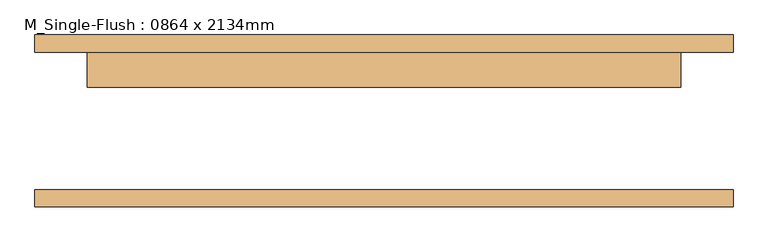
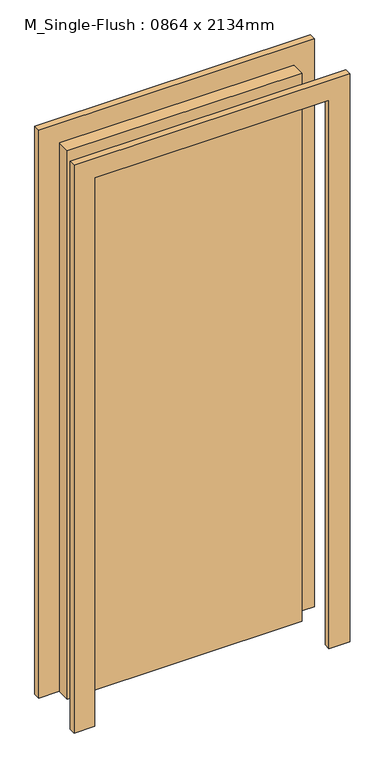
"""IFC4 building model written with IfcOpenShell, lengths in millimetres: door geometry, M_Single-Flush : 0864 x 2134mm."""

from ifc_helpers import new_model, si_unit, frame, origin, origin_with_axes, place, context, project, spatial, polyline, outline, extrude, source, transform, mapped, element, save


def m_single_flush_0864_x_2134mm_5c09ce2c(model_context):
    return source(origin(), model_context, "Body", "SweptSolid", [
        extrude(outline(polyline([(2210.0, -508.0), (0.0, -508.0), (0.0, -432.0), (2134.0, -432.0), (2134.0, 432.0), (0.0, 432.0), (0.0, 508.0), (2210.0, 508.0), (2210.0, -508.0)])), frame((0.0, 100.0, 0.0), z_axis=(0.0, 1.0, 0.0), x_axis=(0.0, 0.0, 1.0)), (0.0, 0.0, 1.0), 25.0),
        extrude(outline(polyline([(2210.0, 508.0), (2210.0, -508.0), (0.0, -508.0), (0.0, -432.0), (2134.0, -432.0), (2134.0, 432.0), (0.0, 432.0), (0.0, 508.0), (2210.0, 508.0)])), frame((0.0, -125.0, 0.0), z_axis=(0.0, 1.0, 0.0), x_axis=(0.0, 0.0, 1.0)), (0.0, 0.0, 1.0), 25.0),
        extrude(outline(polyline([(432.0, 49.0), (-432.0, 49.0), (-432.0, 100.0), (432.0, 100.0), (432.0, 49.0)])), origin_with_axes(), (0.0, 0.0, 1.0), 2134.0),
    ])


if __name__ == "__main__":
    model = new_model("IFC4")
    model_context = context("Model", 3, world=origin())
    ifc_project = project(units=[si_unit("LENGTHUNIT", "METRE", prefix="MILLI")], contexts=[model_context])
    site = spatial("IfcSite", under=ifc_project)
    building = spatial("IfcBuilding", under=site)
    placement = place(None, origin())
    m_single_flush_0864_x_2134mm_shape = m_single_flush_0864_x_2134mm_5c09ce2c(model_context)
    element("IfcDoor", 1, ObjectType="M_Single-Flush : 0864 x 2134mm", at=placement, inside=building, context=model_context, shape_type="MappedRepresentation", body=[
        mapped(m_single_flush_0864_x_2134mm_shape, transform((0.0, 0.0, 0.0), x_axis=(1.0, 0.0, 0.0), y_axis=(0.0, 1.0, 0.0), z_axis=(0.0, 0.0, 1.0))),
    ])
    save(model, "model.ifc")

# Revit data of these elements
# Type "M_Single-Flush : 0864 x 2134mm"
#   Type Mark = "16"
#   Thickness = 51 mm
#   Height = 2134 mm
#   Trim Projection Ext = 25 mm
#   Trim Projection Int = 25 mm
#   Trim Width = 76 mm
#   Width = 864 mm
#   Door Material = Door - Panel
#   Frame Material = Door - Frame
#   Function = (empty or 0)
#   Wall Closure = (empty or 0)
# Element 1 (IfcDoor, "M_Single-Flush : 0864 x 2134mm")
#   Materials on its faces: "Door - Frame", "Door - Panel"
# Materials
#   "Door - Panel": class "Wood", colour RGB 114 82 51, transparency 0
#   "Door - Frame": colour RGB 153 76 43, transparency 0
